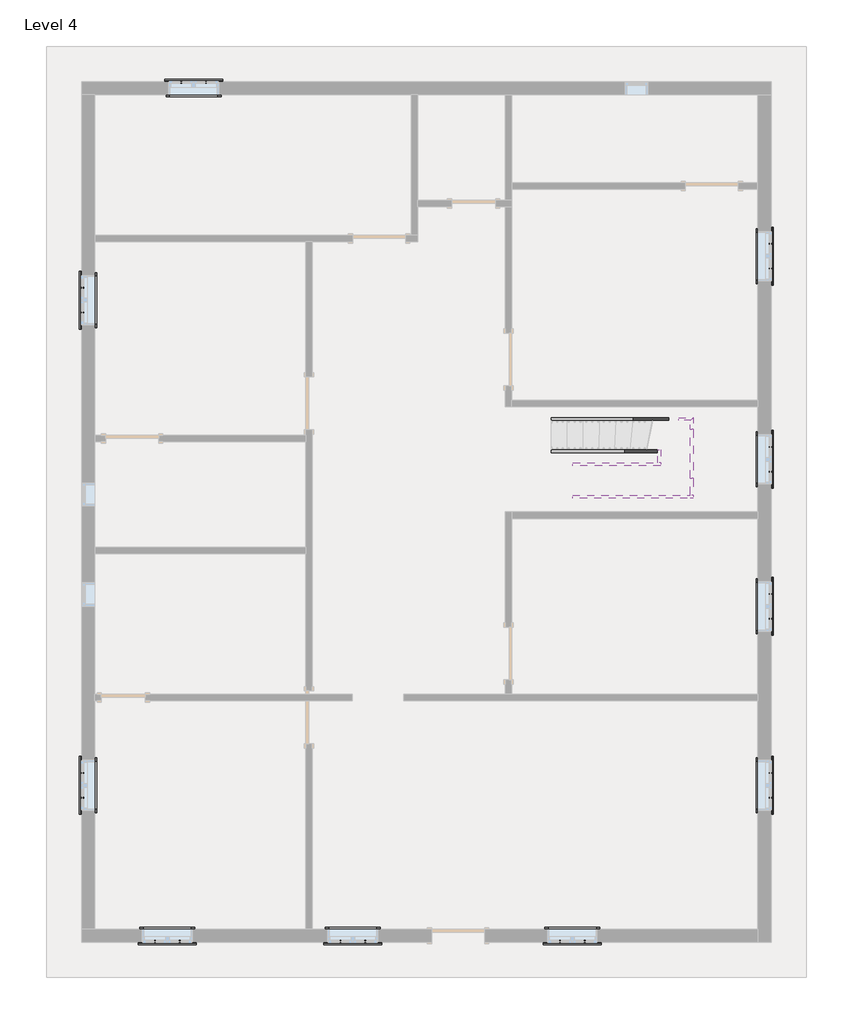
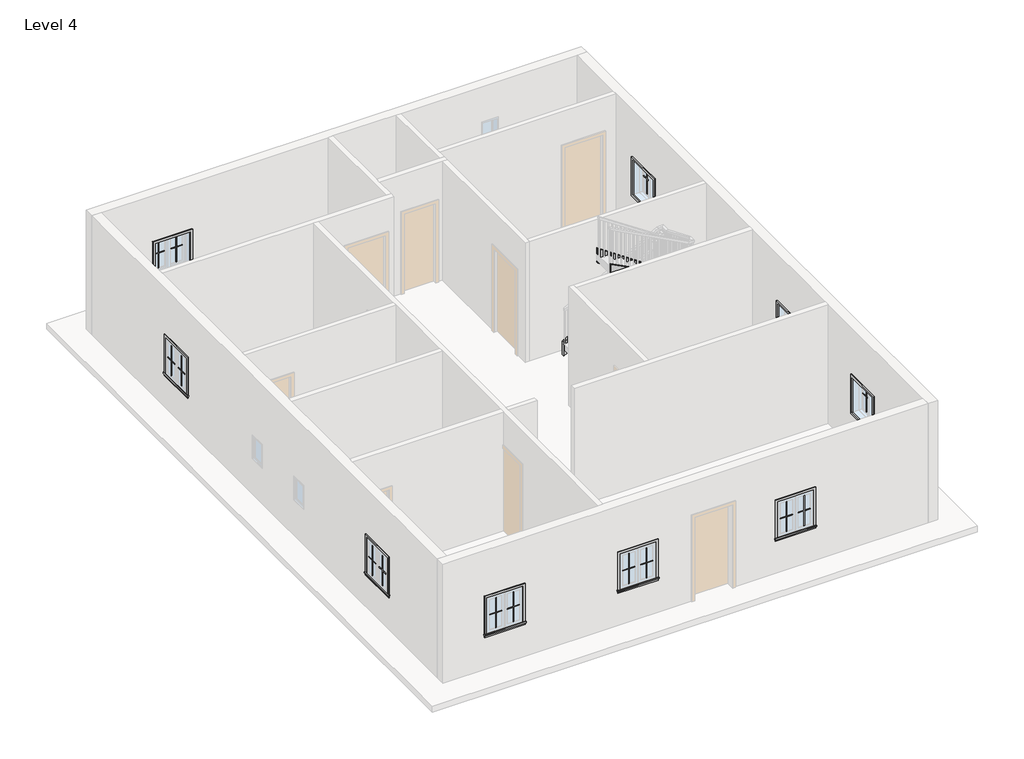
# One storey, part 3 of 3: 40 proxies, 9 members.
"""IFC4 building model written with IfcOpenShell, lengths in millimetres."""

from ifc_helpers import new_model, si_unit, frame, origin, place, context, project, spatial, polyline, outline, extrude, transform, mapped, element, save
from components import muntin_pattern_2x2_muntin_pattern_2x2_b3fe6957, muntin_pattern_2x2_muntin_pattern_2x2_3e0ecaf2, trim_window_exterior_flat_with_sill_41619996, trim_window_interior_flat_picture_frame_51c85655

model = new_model("IFC4")

# Units and contexts
model_context = context("Model", 3, world=origin())
ifc_project = project(units=[si_unit("LENGTHUNIT", "METRE", prefix="MILLI")], contexts=[model_context])

# Site, building, storey
site = spatial("IfcSite", under=ifc_project)
building = spatial("IfcBuilding", under=site)
storey = spatial("IfcBuildingStorey", under=building, Name="Level 4", Elevation=6400.8)

# Proxies
placement = place(None, origin())
muntin_pattern_2x2_muntin_pattern_2x2_shape = muntin_pattern_2x2_muntin_pattern_2x2_b3fe6957(model_context)
element("IfcBuildingElementProxy", 1, Name="Muntin Pattern_2x2 : Muntin Pattern_2x2", ObjectType="Muntin Pattern_2x2 : Muntin Pattern_2x2", at=placement, inside=storey, context=model_context, shape_type="MappedRepresentation", body=[
    mapped(muntin_pattern_2x2_muntin_pattern_2x2_shape, transform((-5581.2368007, 9072.452558, 7385.05), x_axis=(1.0, 0.0, 0.0), y_axis=(0.0, 1.0, 0.0), z_axis=(0.0, 0.0, 1.0))),
])
element("IfcBuildingElementProxy", 2, Name="Muntin Pattern_2x2 : Muntin Pattern_2x2", ObjectType="Muntin Pattern_2x2 : Muntin Pattern_2x2", at=placement, inside=storey, context=model_context, shape_type="MappedRepresentation", body=[
    mapped(muntin_pattern_2x2_muntin_pattern_2x2_shape, transform((-7300.4993007, 5076.715058, 7385.05), x_axis=(0.0, 1.0, 0.0), y_axis=(-1.0, 0.0, 0.0), z_axis=(0.0, 0.0, 1.0))),
])
element("IfcBuildingElementProxy", 3, Name="Muntin Pattern_2x2 : Muntin Pattern_2x2", ObjectType="Muntin Pattern_2x2 : Muntin Pattern_2x2", at=placement, inside=storey, context=model_context, shape_type="MappedRepresentation", body=[
    mapped(muntin_pattern_2x2_muntin_pattern_2x2_shape, transform((4643.8506993, 6267.340058, 7385.05), x_axis=(0.0, -1.0, 0.0), y_axis=(1.0, 0.0, 0.0), z_axis=(0.0, 0.0, 1.0))),
])
element("IfcBuildingElementProxy", 4, Name="Muntin Pattern_2x2 : Muntin Pattern_2x2", ObjectType="Muntin Pattern_2x2 : Muntin Pattern_2x2", at=placement, inside=storey, context=model_context, shape_type="MappedRepresentation", body=[
    mapped(muntin_pattern_2x2_muntin_pattern_2x2_shape, transform((4643.8506993, 2743.090058, 7385.05), x_axis=(0.0, -1.0, 0.0), y_axis=(1.0, 0.0, 0.0), z_axis=(0.0, 0.0, 1.0))),
])
element("IfcBuildingElementProxy", 5, Name="Muntin Pattern_2x2 : Muntin Pattern_2x2", ObjectType="Muntin Pattern_2x2 : Muntin Pattern_2x2", at=placement, inside=storey, context=model_context, shape_type="MappedRepresentation", body=[
    mapped(muntin_pattern_2x2_muntin_pattern_2x2_shape, transform((4643.8506993, 190.390058, 7385.05), x_axis=(0.0, -1.0, 0.0), y_axis=(1.0, 0.0, 0.0), z_axis=(0.0, 0.0, 1.0))),
])
element("IfcBuildingElementProxy", 6, Name="Muntin Pattern_2x2 : Muntin Pattern_2x2", ObjectType="Muntin Pattern_2x2 : Muntin Pattern_2x2", at=placement, inside=storey, context=model_context, shape_type="MappedRepresentation", body=[
    mapped(muntin_pattern_2x2_muntin_pattern_2x2_shape, transform((4643.8506993, -2914.759942, 7385.05), x_axis=(0.0, -1.0, 0.0), y_axis=(1.0, 0.0, 0.0), z_axis=(0.0, 0.0, 1.0))),
])
element("IfcBuildingElementProxy", 7, Name="Muntin Pattern_2x2 : Muntin Pattern_2x2", ObjectType="Muntin Pattern_2x2 : Muntin Pattern_2x2", at=placement, inside=storey, context=model_context, shape_type="MappedRepresentation", body=[
    mapped(muntin_pattern_2x2_muntin_pattern_2x2_shape, transform((1419.6381993, -5843.697442, 7385.05), x_axis=(-1.0, 0.0, 0.0), y_axis=(0.0, -1.0, 0.0), z_axis=(0.0, 0.0, 1.0))),
])
element("IfcBuildingElementProxy", 8, Name="Muntin Pattern_2x2 : Muntin Pattern_2x2", ObjectType="Muntin Pattern_2x2 : Muntin Pattern_2x2", at=placement, inside=storey, context=model_context, shape_type="MappedRepresentation", body=[
    mapped(muntin_pattern_2x2_muntin_pattern_2x2_shape, transform((-2390.3618007, -5843.697442, 7385.05), x_axis=(-1.0, 0.0, 0.0), y_axis=(0.0, -1.0, 0.0), z_axis=(0.0, 0.0, 1.0))),
])
element("IfcBuildingElementProxy", 9, Name="Muntin Pattern_2x2 : Muntin Pattern_2x2", ObjectType="Muntin Pattern_2x2 : Muntin Pattern_2x2", at=placement, inside=storey, context=model_context, shape_type="MappedRepresentation", body=[
    mapped(muntin_pattern_2x2_muntin_pattern_2x2_shape, transform((-5609.8118007, -5843.697442, 7385.05), x_axis=(-1.0, 0.0, 0.0), y_axis=(0.0, -1.0, 0.0), z_axis=(0.0, 0.0, 1.0))),
])
element("IfcBuildingElementProxy", 10, Name="Muntin Pattern_2x2 : Muntin Pattern_2x2", ObjectType="Muntin Pattern_2x2 : Muntin Pattern_2x2", at=placement, inside=storey, context=model_context, shape_type="MappedRepresentation", body=[
    mapped(muntin_pattern_2x2_muntin_pattern_2x2_shape, transform((-7300.4993007, -3343.384942, 7385.05), x_axis=(0.0, 1.0, 0.0), y_axis=(-1.0, 0.0, 0.0), z_axis=(0.0, 0.0, 1.0))),
])
muntin_pattern_2x2_muntin_pattern_2x2_2_shape = muntin_pattern_2x2_muntin_pattern_2x2_3e0ecaf2(model_context)
element("IfcBuildingElementProxy", 11, Name="Muntin Pattern_2x2 : Muntin Pattern_2x2", ObjectType="Muntin Pattern_2x2 : Muntin Pattern_2x2", at=placement, inside=storey, context=model_context, shape_type="MappedRepresentation", body=[
    mapped(muntin_pattern_2x2_muntin_pattern_2x2_2_shape, transform((-5152.6118007, 9072.452558, 7385.05), x_axis=(-1.0, 0.0, 0.0), y_axis=(0.0, -1.0, 0.0), z_axis=(0.0, 0.0, 1.0))),
])
element("IfcBuildingElementProxy", 12, Name="Muntin Pattern_2x2 : Muntin Pattern_2x2", ObjectType="Muntin Pattern_2x2 : Muntin Pattern_2x2", at=placement, inside=storey, context=model_context, shape_type="MappedRepresentation", body=[
    mapped(muntin_pattern_2x2_muntin_pattern_2x2_2_shape, transform((-7300.4993007, 5505.340058, 7385.05), x_axis=(0.0, -1.0, 0.0), y_axis=(1.0, 0.0, 0.0), z_axis=(0.0, 0.0, 1.0))),
])
element("IfcBuildingElementProxy", 13, Name="Muntin Pattern_2x2 : Muntin Pattern_2x2", ObjectType="Muntin Pattern_2x2 : Muntin Pattern_2x2", at=placement, inside=storey, context=model_context, shape_type="MappedRepresentation", body=[
    mapped(muntin_pattern_2x2_muntin_pattern_2x2_2_shape, transform((4643.8506993, 5838.715058, 7385.05), x_axis=(0.0, 1.0, 0.0), y_axis=(-1.0, 0.0, 0.0), z_axis=(0.0, 0.0, 1.0))),
])
element("IfcBuildingElementProxy", 14, Name="Muntin Pattern_2x2 : Muntin Pattern_2x2", ObjectType="Muntin Pattern_2x2 : Muntin Pattern_2x2", at=placement, inside=storey, context=model_context, shape_type="MappedRepresentation", body=[
    mapped(muntin_pattern_2x2_muntin_pattern_2x2_2_shape, transform((4643.8506993, 2314.465058, 7385.05), x_axis=(0.0, 1.0, 0.0), y_axis=(-1.0, 0.0, 0.0), z_axis=(0.0, 0.0, 1.0))),
])
element("IfcBuildingElementProxy", 15, Name="Muntin Pattern_2x2 : Muntin Pattern_2x2", ObjectType="Muntin Pattern_2x2 : Muntin Pattern_2x2", at=placement, inside=storey, context=model_context, shape_type="MappedRepresentation", body=[
    mapped(muntin_pattern_2x2_muntin_pattern_2x2_2_shape, transform((4643.8506993, -238.234942, 7385.05), x_axis=(0.0, 1.0, 0.0), y_axis=(-1.0, 0.0, 0.0), z_axis=(0.0, 0.0, 1.0))),
])
element("IfcBuildingElementProxy", 16, Name="Muntin Pattern_2x2 : Muntin Pattern_2x2", ObjectType="Muntin Pattern_2x2 : Muntin Pattern_2x2", at=placement, inside=storey, context=model_context, shape_type="MappedRepresentation", body=[
    mapped(muntin_pattern_2x2_muntin_pattern_2x2_2_shape, transform((4643.8506993, -3343.384942, 7385.05), x_axis=(0.0, 1.0, 0.0), y_axis=(-1.0, 0.0, 0.0), z_axis=(0.0, 0.0, 1.0))),
])
element("IfcBuildingElementProxy", 17, Name="Muntin Pattern_2x2 : Muntin Pattern_2x2", ObjectType="Muntin Pattern_2x2 : Muntin Pattern_2x2", at=placement, inside=storey, context=model_context, shape_type="MappedRepresentation", body=[
    mapped(muntin_pattern_2x2_muntin_pattern_2x2_2_shape, transform((991.0131993, -5843.697442, 7385.05), x_axis=(1.0, 0.0, 0.0), y_axis=(0.0, 1.0, 0.0), z_axis=(0.0, 0.0, 1.0))),
])
element("IfcBuildingElementProxy", 18, Name="Muntin Pattern_2x2 : Muntin Pattern_2x2", ObjectType="Muntin Pattern_2x2 : Muntin Pattern_2x2", at=placement, inside=storey, context=model_context, shape_type="MappedRepresentation", body=[
    mapped(muntin_pattern_2x2_muntin_pattern_2x2_2_shape, transform((-2818.9868007, -5843.697442, 7385.05), x_axis=(1.0, 0.0, 0.0), y_axis=(0.0, 1.0, 0.0), z_axis=(0.0, 0.0, 1.0))),
])
element("IfcBuildingElementProxy", 19, Name="Muntin Pattern_2x2 : Muntin Pattern_2x2", ObjectType="Muntin Pattern_2x2 : Muntin Pattern_2x2", at=placement, inside=storey, context=model_context, shape_type="MappedRepresentation", body=[
    mapped(muntin_pattern_2x2_muntin_pattern_2x2_2_shape, transform((-6038.4368007, -5843.697442, 7385.05), x_axis=(1.0, 0.0, 0.0), y_axis=(0.0, 1.0, 0.0), z_axis=(0.0, 0.0, 1.0))),
])
element("IfcBuildingElementProxy", 20, Name="Muntin Pattern_2x2 : Muntin Pattern_2x2", ObjectType="Muntin Pattern_2x2 : Muntin Pattern_2x2", at=placement, inside=storey, context=model_context, shape_type="MappedRepresentation", body=[
    mapped(muntin_pattern_2x2_muntin_pattern_2x2_2_shape, transform((-7300.4993007, -2914.759942, 7385.05), x_axis=(0.0, -1.0, 0.0), y_axis=(1.0, 0.0, 0.0), z_axis=(0.0, 0.0, 1.0))),
])
trim_window_exterior_flat_with_sill_shape = trim_window_exterior_flat_with_sill_41619996(model_context)
element("IfcBuildingElementProxy", 21, Name="Trim-Window-Exterior-Flat : with Sill", ObjectType="Trim-Window-Exterior-Flat : with Sill", at=placement, inside=storey, context=model_context, shape_type="MappedRepresentation", body=[
    mapped(trim_window_exterior_flat_with_sill_shape, transform((-5366.9243007, 9081.977558, 8229.6), x_axis=(-1.0, 0.0, 0.0), y_axis=(0.0, 0.0, 1.0), z_axis=(0.0, 1.0, 0.0))),
])
element("IfcBuildingElementProxy", 22, Name="Trim-Window-Exterior-Flat : with Sill", ObjectType="Trim-Window-Exterior-Flat : with Sill", at=placement, inside=storey, context=model_context, shape_type="MappedRepresentation", body=[
    mapped(trim_window_exterior_flat_with_sill_shape, transform((-7310.0243007, 5291.027558, 8229.6), x_axis=(0.0, -1.0, 0.0), y_axis=(0.0, 0.0, 1.0), z_axis=(-1.0, 0.0, 0.0))),
])
element("IfcBuildingElementProxy", 23, Name="Trim-Window-Exterior-Flat : with Sill", ObjectType="Trim-Window-Exterior-Flat : with Sill", at=placement, inside=storey, context=model_context, shape_type="MappedRepresentation", body=[
    mapped(trim_window_exterior_flat_with_sill_shape, transform((4653.3756993, 6053.027558, 8229.6), x_axis=(0.0, 1.0, 0.0), y_axis=(0.0, 0.0, 1.0), z_axis=(1.0, 0.0, 0.0))),
])
element("IfcBuildingElementProxy", 24, Name="Trim-Window-Exterior-Flat : with Sill", ObjectType="Trim-Window-Exterior-Flat : with Sill", at=placement, inside=storey, context=model_context, shape_type="MappedRepresentation", body=[
    mapped(trim_window_exterior_flat_with_sill_shape, transform((4653.3756993, 2528.777558, 8229.6), x_axis=(0.0, 1.0, 0.0), y_axis=(0.0, 0.0, 1.0), z_axis=(1.0, 0.0, 0.0))),
])
element("IfcBuildingElementProxy", 25, Name="Trim-Window-Exterior-Flat : with Sill", ObjectType="Trim-Window-Exterior-Flat : with Sill", at=placement, inside=storey, context=model_context, shape_type="MappedRepresentation", body=[
    mapped(trim_window_exterior_flat_with_sill_shape, transform((4653.3756993, -23.922442, 8229.6), x_axis=(0.0, 1.0, 0.0), y_axis=(0.0, 0.0, 1.0), z_axis=(1.0, 0.0, 0.0))),
])
element("IfcBuildingElementProxy", 26, Name="Trim-Window-Exterior-Flat : with Sill", ObjectType="Trim-Window-Exterior-Flat : with Sill", at=placement, inside=storey, context=model_context, shape_type="MappedRepresentation", body=[
    mapped(trim_window_exterior_flat_with_sill_shape, transform((4653.3756993, -3129.072442, 8229.6), x_axis=(0.0, 1.0, 0.0), y_axis=(0.0, 0.0, 1.0), z_axis=(1.0, 0.0, 0.0))),
])
element("IfcBuildingElementProxy", 27, Name="Trim-Window-Exterior-Flat : with Sill", ObjectType="Trim-Window-Exterior-Flat : with Sill", at=placement, inside=storey, context=model_context, shape_type="MappedRepresentation", body=[
    mapped(trim_window_exterior_flat_with_sill_shape, transform((1205.3256993, -5853.222442, 8229.6), x_axis=(1.0, 0.0, 0.0), y_axis=(0.0, 0.0, 1.0), z_axis=(0.0, -1.0, 0.0))),
])
element("IfcBuildingElementProxy", 28, Name="Trim-Window-Exterior-Flat : with Sill", ObjectType="Trim-Window-Exterior-Flat : with Sill", at=placement, inside=storey, context=model_context, shape_type="MappedRepresentation", body=[
    mapped(trim_window_exterior_flat_with_sill_shape, transform((-2604.6743007, -5853.222442, 8229.6), x_axis=(1.0, 0.0, 0.0), y_axis=(0.0, 0.0, 1.0), z_axis=(0.0, -1.0, 0.0))),
])
element("IfcBuildingElementProxy", 29, Name="Trim-Window-Exterior-Flat : with Sill", ObjectType="Trim-Window-Exterior-Flat : with Sill", at=placement, inside=storey, context=model_context, shape_type="MappedRepresentation", body=[
    mapped(trim_window_exterior_flat_with_sill_shape, transform((-5824.1243007, -5853.222442, 8229.6), x_axis=(1.0, 0.0, 0.0), y_axis=(0.0, 0.0, 1.0), z_axis=(0.0, -1.0, 0.0))),
])
element("IfcBuildingElementProxy", 30, Name="Trim-Window-Exterior-Flat : with Sill", ObjectType="Trim-Window-Exterior-Flat : with Sill", at=placement, inside=storey, context=model_context, shape_type="MappedRepresentation", body=[
    mapped(trim_window_exterior_flat_with_sill_shape, transform((-7310.0243007, -3129.072442, 8229.6), x_axis=(0.0, -1.0, 0.0), y_axis=(0.0, 0.0, 1.0), z_axis=(-1.0, 0.0, 0.0))),
])
trim_window_interior_flat_picture_frame_shape = trim_window_interior_flat_picture_frame_51c85655(model_context)
element("IfcBuildingElementProxy", 31, Name="Trim-Window-Interior-Flat : Picture Frame", ObjectType="Trim-Window-Interior-Flat : Picture Frame", at=placement, inside=storey, context=model_context, shape_type="MappedRepresentation", body=[
    mapped(trim_window_interior_flat_picture_frame_shape, transform((-5366.9243007, 8853.377558, 8229.6), x_axis=(1.0, 0.0, 0.0), y_axis=(0.0, 0.0, 1.0), z_axis=(0.0, -1.0, 0.0))),
])
element("IfcBuildingElementProxy", 32, Name="Trim-Window-Interior-Flat : Picture Frame", ObjectType="Trim-Window-Interior-Flat : Picture Frame", at=placement, inside=storey, context=model_context, shape_type="MappedRepresentation", body=[
    mapped(trim_window_interior_flat_picture_frame_shape, transform((-7081.4243007, 5291.027558, 8229.6), x_axis=(0.0, 1.0, 0.0), y_axis=(0.0, 0.0, 1.0), z_axis=(1.0, 0.0, 0.0))),
])
element("IfcBuildingElementProxy", 33, Name="Trim-Window-Interior-Flat : Picture Frame", ObjectType="Trim-Window-Interior-Flat : Picture Frame", at=placement, inside=storey, context=model_context, shape_type="MappedRepresentation", body=[
    mapped(trim_window_interior_flat_picture_frame_shape, transform((4424.7756993, 6053.027558, 8229.6), x_axis=(0.0, -1.0, 0.0), y_axis=(0.0, 0.0, 1.0), z_axis=(-1.0, 0.0, 0.0))),
])
element("IfcBuildingElementProxy", 34, Name="Trim-Window-Interior-Flat : Picture Frame", ObjectType="Trim-Window-Interior-Flat : Picture Frame", at=placement, inside=storey, context=model_context, shape_type="MappedRepresentation", body=[
    mapped(trim_window_interior_flat_picture_frame_shape, transform((4424.7756993, 2528.777558, 8229.6), x_axis=(0.0, -1.0, 0.0), y_axis=(0.0, 0.0, 1.0), z_axis=(-1.0, 0.0, 0.0))),
])
element("IfcBuildingElementProxy", 35, Name="Trim-Window-Interior-Flat : Picture Frame", ObjectType="Trim-Window-Interior-Flat : Picture Frame", at=placement, inside=storey, context=model_context, shape_type="MappedRepresentation", body=[
    mapped(trim_window_interior_flat_picture_frame_shape, transform((4424.7756993, -23.922442, 8229.6), x_axis=(0.0, -1.0, 0.0), y_axis=(0.0, 0.0, 1.0), z_axis=(-1.0, 0.0, 0.0))),
])
element("IfcBuildingElementProxy", 36, Name="Trim-Window-Interior-Flat : Picture Frame", ObjectType="Trim-Window-Interior-Flat : Picture Frame", at=placement, inside=storey, context=model_context, shape_type="MappedRepresentation", body=[
    mapped(trim_window_interior_flat_picture_frame_shape, transform((4424.7756993, -3129.072442, 8229.6), x_axis=(0.0, -1.0, 0.0), y_axis=(0.0, 0.0, 1.0), z_axis=(-1.0, 0.0, 0.0))),
])
element("IfcBuildingElementProxy", 37, Name="Trim-Window-Interior-Flat : Picture Frame", ObjectType="Trim-Window-Interior-Flat : Picture Frame", at=placement, inside=storey, context=model_context, shape_type="MappedRepresentation", body=[
    mapped(trim_window_interior_flat_picture_frame_shape, transform((1205.3256993, -5624.622442, 8229.6), x_axis=(-1.0, 0.0, 0.0), y_axis=(0.0, 0.0, 1.0), z_axis=(0.0, 1.0, 0.0))),
])
element("IfcBuildingElementProxy", 38, Name="Trim-Window-Interior-Flat : Picture Frame", ObjectType="Trim-Window-Interior-Flat : Picture Frame", at=placement, inside=storey, context=model_context, shape_type="MappedRepresentation", body=[
    mapped(trim_window_interior_flat_picture_frame_shape, transform((-2604.6743007, -5624.622442, 8229.6), x_axis=(-1.0, 0.0, 0.0), y_axis=(0.0, 0.0, 1.0), z_axis=(0.0, 1.0, 0.0))),
])
element("IfcBuildingElementProxy", 39, Name="Trim-Window-Interior-Flat : Picture Frame", ObjectType="Trim-Window-Interior-Flat : Picture Frame", at=placement, inside=storey, context=model_context, shape_type="MappedRepresentation", body=[
    mapped(trim_window_interior_flat_picture_frame_shape, transform((-5824.1243007, -5624.622442, 8229.6), x_axis=(-1.0, 0.0, 0.0), y_axis=(0.0, 0.0, 1.0), z_axis=(0.0, 1.0, 0.0))),
])
element("IfcBuildingElementProxy", 40, Name="Trim-Window-Interior-Flat : Picture Frame", ObjectType="Trim-Window-Interior-Flat : Picture Frame", at=placement, inside=storey, context=model_context, shape_type="MappedRepresentation", body=[
    mapped(trim_window_interior_flat_picture_frame_shape, transform((-7081.4243007, -3129.072442, 8229.6), x_axis=(0.0, 1.0, 0.0), y_axis=(0.0, 0.0, 1.0), z_axis=(1.0, 0.0, 0.0))),
])

# Members
element("IfcMember", 41, ObjectType="Stringer - 2\" Width", at=placement, inside=storey, context=model_context, shape_type="SweptSolid", body=[
    extrude(outline(polyline([(6789.2746569, 838.4202681), (6438.6072902, 838.4202681), (7698.2160324, 3052.6525996), (8048.8833991, 3052.6525996), (6789.2746569, 838.4202681)])), frame((0.0, 3202.4524989, 0.0), z_axis=(0.0, 1.0, 0.0), x_axis=(0.0, 0.0, 1.0)), (0.0, 0.0, 1.0), 50.8),
])
element("IfcMember", 42, ObjectType="Stringer - 2\" Width", at=placement, inside=storey, context=model_context, shape_type="SweptSolid", body=[
    extrude(outline(polyline([(3052.6525996, 3202.4524989), (3052.6525996, 3253.2524989), (3298.782332, 3253.2524989), (3247.982332, 3202.4524989), (3052.6525996, 3202.4524989)])), frame((0.0, 0.0, 7698.2160324), z_axis=(0.0, 0.0, 1.0), x_axis=(1.0, 0.0, 0.0)), (0.0, 0.0, 1.0), 350.6673667),
])
element("IfcMember", 43, ObjectType="Stringer - 2\" Width", at=placement, inside=storey, context=model_context, shape_type="SweptSolid", body=[
    extrude(outline(polyline([(3247.982332, 3202.4524989), (3298.782332, 3253.2524989), (3298.782332, 3048.1586437), (3247.982332, 3048.1586437), (3247.982332, 3202.4524989)])), frame((0.0, 0.0, 7698.2160324), z_axis=(0.0, 0.0, 1.0), x_axis=(1.0, 0.0, 0.0)), (0.0, 0.0, 1.0), 350.6673667),
])
element("IfcMember", 44, ObjectType="Stringer - 2\" Width", at=placement, inside=storey, context=model_context, shape_type="SweptSolid", body=[
    extrude(outline(polyline([(3048.1586437, 8048.8833991), (3048.1586437, 7698.2160324), (2198.376501, 8053.7779505), (2198.376501, 8404.4453172), (3048.1586437, 8048.8833991)])), frame((3247.982332, 0.0, 0.0), z_axis=(1.0, 0.0, 0.0), x_axis=(0.0, 1.0, 0.0)), (0.0, 0.0, 1.0), 50.8),
])
element("IfcMember", 45, ObjectType="Stringer - 2\" Width", at=placement, inside=storey, context=model_context, shape_type="SweptSolid", body=[
    extrude(outline(polyline([(3247.982332, 2198.376501), (3298.782332, 2198.376501), (3298.782332, 1905.9026171), (3247.982332, 1905.9026171), (3247.982332, 2198.376501)])), frame((0.0, 0.0, 8062.7761112), z_axis=(0.0, 0.0, 1.0), x_axis=(1.0, 0.0, 0.0)), (0.0, 0.0, 1.0), 330.4053693),
])
element("IfcMember", 46, ObjectType="Stringer - 2\" Width", at=placement, inside=storey, context=model_context, shape_type="SweptSolid", body=[
    extrude(outline(polyline([(6774.8558321, 838.4202681), (6411.9163437, 838.4202681), (7607.9401496, 2688.6073911), (7970.8796379, 2688.6073911), (6774.8558321, 838.4202681)])), frame((0.0, 2643.077558, 0.0), z_axis=(0.0, 1.0, 0.0), x_axis=(0.0, 0.0, 1.0)), (0.0, 0.0, 1.0), 50.8),
])
element("IfcMember", 47, ObjectType="Stringer - 2\" Width", at=placement, inside=storey, context=model_context, shape_type="SweptSolid", body=[
    extrude(outline(polyline([(2693.877558, 8138.2149577), (2693.877558, 7690.9996268), (2465.277558, 7936.4439445), (2465.277558, 8383.6592754), (2693.877558, 8138.2149577)])), frame((2688.6073911, 0.0, 0.0), z_axis=(1.0, 0.0, 0.0), x_axis=(0.0, 1.0, 0.0)), (0.0, 0.0, 1.0), 50.8),
])
element("IfcMember", 48, ObjectType="Stringer - 2\" Width", at=placement, inside=storey, context=model_context, shape_type="SweptSolid", body=[
    extrude(outline(polyline([(8101.5150039, 2739.4073911), (8471.491358, 2739.4073911), (9522.6229383, 1211.6756993), (9152.6465842, 1211.6756993), (8101.5150039, 2739.4073911)])), frame((0.0, 2414.477558, 0.0), z_axis=(0.0, 1.0, 0.0), x_axis=(0.0, 0.0, 1.0)), (0.0, 0.0, 1.0), 50.8),
])
element("IfcMember", 49, ObjectType="Stringer - 2\" Width", at=placement, inside=storey, context=model_context, shape_type="SweptSolid", body=[
    extrude(outline(polyline([(8088.3814805, 3298.782332), (8366.7410006, 3298.782332), (9453.042202, 1211.6756993), (9122.6368327, 1211.6756993), (8088.3814805, 3198.7868271), (8088.3814805, 3298.782332)])), frame((0.0, 1855.1026171, 0.0), z_axis=(0.0, 1.0, 0.0), x_axis=(0.0, 0.0, 1.0)), (0.0, 0.0, 1.0), 50.8),
])

save(model, "model.ifc")

# Revit data of these elements
# Type "Muntin Pattern_2x2 : Muntin Pattern_2x2"
#   Width [instance default] = 4' - 0"
#   Thickness = 0' - 0 1/2"
#   Height [instance default] = 4' - 0"
#   Distance = 0' - 0 3/4"
#   Interior Material [instance default] = none
#   Exterior Material [instance default] = none
#   Default Elevation = 0
# Type "Trim-Window-Exterior-Flat : with Sill"
#   Trim Width = 0' - 2 1/4"
#   Trim Thickness_Picture Frame = 0' - 1 1/4"
#   Trim Thickness_with Sill = 0' - 0 3/4"
#   Sill Thickness = 0' - 1 1/4"
#   Opening Width [instance default] = 2' - 0"
#   Opening Height [instance default] = 3' - 0"
#   Default Elevation = 4' - 0"
#   Sill = yes
#   Picture Frame = no
#   Trim Material [instance default] = none
# Type "Trim-Window-Interior-Flat : Picture Frame"
#   Trim Thickness_Picture Frame = 0' - 1 1/4"
#   Trim Width = 0' - 2 1/4"
#   Trim Thickness_with Sill = 0' - 0 3/4"
#   Sill Thickness = 0' - 1 1/4"
#   Opening Width [instance default] = 2' - 0"
#   Opening Height [instance default] = 3' - 0"
#   Default Elevation = 4' - 0"
#   Sill = no
#   Picture Frame = yes
#   Trim Material [instance default] = none
# Elements 1, 2, 3, 4, 5, 6, 7, 8, 9, 10, 11, 12, 13, 14, 15, 16, 17, 18, 19, 20 (IfcBuildingElementProxy, "Muntin Pattern_2x2 : Muntin Pattern_2x2")
#   Width = 0' - 11 5/8"
#   Height = 2' - 6 1/2"
#   Interior Material = Wood - Stained
#   Exterior Material = Clad - White
#   Phase Created = New Construction
#   Materials on its faces: "Clad - White", "Wood - Stained"
# Elements 21, 22, 23, 24, 25, 26, 27, 28, 29, 30 (IfcBuildingElementProxy, "Trim-Window-Exterior-Flat : with Sill")
#   Opening Width = 2' - 10"
#   Opening Height = 3' - 0"
#   Trim Material = Clad - White
#   Phase Created = New Construction
#   Materials on its faces: "Clad - White"
# Elements 31, 32, 33, 34, 35, 36, 37, 38, 39, 40 (IfcBuildingElementProxy, "Trim-Window-Interior-Flat : Picture Frame")
#   Opening Width = 2' - 10"
#   Opening Height = 3' - 0"
#   Trim Material = Wood - Stained
#   Phase Created = New Construction
#   Materials on its faces: "Wood - Stained"
# Elements 41, 42, 43, 44, 45, 46, 47, 48, 49 (IfcMember, "Stringer - 2\" Width")
#   Phase Created = New Construction
# Materials
#   "Clad - White": class "Wood", colour RGB 242 242 238, transparency 0, Cost = 0
#   "Wood - Stained": class "Wood", colour RGB 224 178 126, transparency 0, Cost = 0
